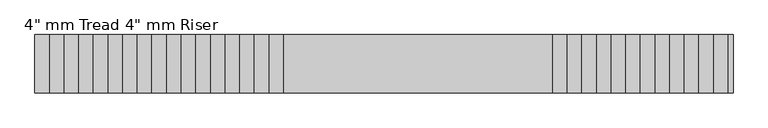
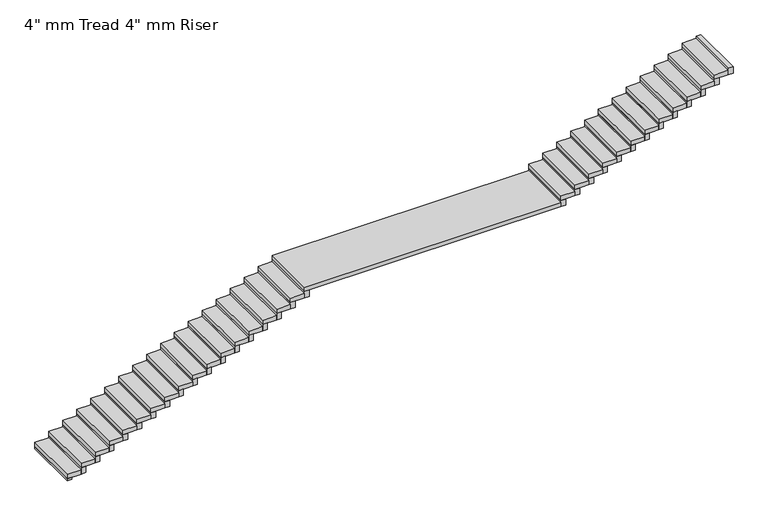
"""IFC4 building model written with IfcOpenShell, lengths in millimetres: stair flight geometry."""

from ifc_helpers import new_model, si_unit, frame, origin, origin_with_axes, place, context, project, spatial, polyline, outline, extrude, source, transform, mapped, element, save


def stair_flight_c4523bda(model_context):
    return source(origin(), model_context, "Body", "SweptSolid", [
        extrude(outline(polyline([(18088.5587563, -31336.2205555), (17986.9587563, -31336.2205555), (17986.9587563, -30117.0205555), (18088.5587563, -30117.0205555), (18088.5587563, -31336.2205555)])), origin_with_axes(), (0.0, 0.0, 1.0), 45.883871),
        extrude(outline(polyline([(18291.7587563, -30117.0205555), (18291.7587563, -31336.2205555), (17986.9587563, -31336.2205555), (17986.9587563, -30117.0205555), (18291.7587563, -30117.0205555)])), frame((0.0, 0.0, 45.883871), z_axis=(0.0, 0.0, 1.0), x_axis=(1.0, 0.0, 0.0)), (0.0, 0.0, 1.0), 101.6),
        extrude(outline(polyline([(18393.3587563, -31336.2205555), (18291.7587563, -31336.2205555), (18291.7587563, -30117.0205555), (18393.3587563, -30117.0205555), (18393.3587563, -31336.2205555)])), frame((0.0, 0.0, 45.883871), z_axis=(0.0, 0.0, 1.0), x_axis=(1.0, 0.0, 0.0)), (0.0, 0.0, 1.0), 147.483871),
        extrude(outline(polyline([(18596.5587563, -30117.0205555), (18596.5587563, -31336.2205555), (18291.7587563, -31336.2205555), (18291.7587563, -30117.0205555), (18596.5587563, -30117.0205555)])), frame((0.0, 0.0, 193.3677419), z_axis=(0.0, 0.0, 1.0), x_axis=(1.0, 0.0, 0.0)), (0.0, 0.0, 1.0), 101.6),
        extrude(outline(polyline([(18698.1587563, -31336.2205555), (18596.5587563, -31336.2205555), (18596.5587563, -30117.0205555), (18698.1587563, -30117.0205555), (18698.1587563, -31336.2205555)])), frame((0.0, 0.0, 193.3677419), z_axis=(0.0, 0.0, 1.0), x_axis=(1.0, 0.0, 0.0)), (0.0, 0.0, 1.0), 147.483871),
        extrude(outline(polyline([(18901.3587563, -30117.0205555), (18901.3587563, -31336.2205555), (18596.5587563, -31336.2205555), (18596.5587563, -30117.0205555), (18901.3587563, -30117.0205555)])), frame((0.0, 0.0, 340.8516129), z_axis=(0.0, 0.0, 1.0), x_axis=(1.0, 0.0, 0.0)), (0.0, 0.0, 1.0), 101.6),
        extrude(outline(polyline([(19002.9587563, -31336.2205555), (18901.3587563, -31336.2205555), (18901.3587563, -30117.0205555), (19002.9587563, -30117.0205555), (19002.9587563, -31336.2205555)])), frame((0.0, 0.0, 340.8516129), z_axis=(0.0, 0.0, 1.0), x_axis=(1.0, 0.0, 0.0)), (0.0, 0.0, 1.0), 147.483871),
        extrude(outline(polyline([(19206.1587563, -30117.0205555), (19206.1587563, -31336.2205555), (18901.3587563, -31336.2205555), (18901.3587563, -30117.0205555), (19206.1587563, -30117.0205555)])), frame((0.0, 0.0, 488.3354839), z_axis=(0.0, 0.0, 1.0), x_axis=(1.0, 0.0, 0.0)), (0.0, 0.0, 1.0), 101.6),
        extrude(outline(polyline([(19307.7587563, -31336.2205555), (19206.1587563, -31336.2205555), (19206.1587563, -30117.0205555), (19307.7587563, -30117.0205555), (19307.7587563, -31336.2205555)])), frame((0.0, 0.0, 488.3354839), z_axis=(0.0, 0.0, 1.0), x_axis=(1.0, 0.0, 0.0)), (0.0, 0.0, 1.0), 147.483871),
        extrude(outline(polyline([(19510.9587563, -30117.0205555), (19510.9587563, -31336.2205555), (19206.1587563, -31336.2205555), (19206.1587563, -30117.0205555), (19510.9587563, -30117.0205555)])), frame((0.0, 0.0, 635.8193548), z_axis=(0.0, 0.0, 1.0), x_axis=(1.0, 0.0, 0.0)), (0.0, 0.0, 1.0), 101.6),
        extrude(outline(polyline([(19612.5587563, -31336.2205555), (19510.9587563, -31336.2205555), (19510.9587563, -30117.0205555), (19612.5587563, -30117.0205555), (19612.5587563, -31336.2205555)])), frame((0.0, 0.0, 635.8193548), z_axis=(0.0, 0.0, 1.0), x_axis=(1.0, 0.0, 0.0)), (0.0, 0.0, 1.0), 147.483871),
        extrude(outline(polyline([(19815.7587563, -30117.0205555), (19815.7587563, -31336.2205555), (19510.9587563, -31336.2205555), (19510.9587563, -30117.0205555), (19815.7587563, -30117.0205555)])), frame((0.0, 0.0, 783.3032258), z_axis=(0.0, 0.0, 1.0), x_axis=(1.0, 0.0, 0.0)), (0.0, 0.0, 1.0), 101.6),
        extrude(outline(polyline([(19917.3587563, -31336.2205555), (19815.7587563, -31336.2205555), (19815.7587563, -30117.0205555), (19917.3587563, -30117.0205555), (19917.3587563, -31336.2205555)])), frame((0.0, 0.0, 783.3032258), z_axis=(0.0, 0.0, 1.0), x_axis=(1.0, 0.0, 0.0)), (0.0, 0.0, 1.0), 147.483871),
        extrude(outline(polyline([(20120.5587563, -30117.0205555), (20120.5587563, -31336.2205555), (19815.7587563, -31336.2205555), (19815.7587563, -30117.0205555), (20120.5587563, -30117.0205555)])), frame((0.0, 0.0, 930.7870968), z_axis=(0.0, 0.0, 1.0), x_axis=(1.0, 0.0, 0.0)), (0.0, 0.0, 1.0), 101.6),
        extrude(outline(polyline([(20222.1587563, -31336.2205555), (20120.5587563, -31336.2205555), (20120.5587563, -30117.0205555), (20222.1587563, -30117.0205555), (20222.1587563, -31336.2205555)])), frame((0.0, 0.0, 930.7870968), z_axis=(0.0, 0.0, 1.0), x_axis=(1.0, 0.0, 0.0)), (0.0, 0.0, 1.0), 147.483871),
        extrude(outline(polyline([(20425.3587563, -30117.0205555), (20425.3587563, -31336.2205555), (20120.5587563, -31336.2205555), (20120.5587563, -30117.0205555), (20425.3587563, -30117.0205555)])), frame((0.0, 0.0, 1078.2709677), z_axis=(0.0, 0.0, 1.0), x_axis=(1.0, 0.0, 0.0)), (0.0, 0.0, 1.0), 101.6),
        extrude(outline(polyline([(20526.9587563, -31336.2205555), (20425.3587563, -31336.2205555), (20425.3587563, -30117.0205555), (20526.9587563, -30117.0205555), (20526.9587563, -31336.2205555)])), frame((0.0, 0.0, 1078.2709677), z_axis=(0.0, 0.0, 1.0), x_axis=(1.0, 0.0, 0.0)), (0.0, 0.0, 1.0), 147.483871),
        extrude(outline(polyline([(20730.1587563, -30117.0205555), (20730.1587563, -31336.2205555), (20425.3587563, -31336.2205555), (20425.3587563, -30117.0205555), (20730.1587563, -30117.0205555)])), frame((0.0, 0.0, 1225.7548387), z_axis=(0.0, 0.0, 1.0), x_axis=(1.0, 0.0, 0.0)), (0.0, 0.0, 1.0), 101.6),
        extrude(outline(polyline([(20831.7587563, -31336.2205555), (20730.1587563, -31336.2205555), (20730.1587563, -30117.0205555), (20831.7587563, -30117.0205555), (20831.7587563, -31336.2205555)])), frame((0.0, 0.0, 1225.7548387), z_axis=(0.0, 0.0, 1.0), x_axis=(1.0, 0.0, 0.0)), (0.0, 0.0, 1.0), 147.483871),
        extrude(outline(polyline([(21034.9587563, -30117.0205555), (21034.9587563, -31336.2205555), (20730.1587563, -31336.2205555), (20730.1587563, -30117.0205555), (21034.9587563, -30117.0205555)])), frame((0.0, 0.0, 1373.2387097), z_axis=(0.0, 0.0, 1.0), x_axis=(1.0, 0.0, 0.0)), (0.0, 0.0, 1.0), 101.6),
        extrude(outline(polyline([(21136.5587563, -31336.2205555), (21034.9587563, -31336.2205555), (21034.9587563, -30117.0205555), (21136.5587563, -30117.0205555), (21136.5587563, -31336.2205555)])), frame((0.0, 0.0, 1373.2387097), z_axis=(0.0, 0.0, 1.0), x_axis=(1.0, 0.0, 0.0)), (0.0, 0.0, 1.0), 147.483871),
        extrude(outline(polyline([(21339.7587563, -30117.0205555), (21339.7587563, -31336.2205555), (21034.9587563, -31336.2205555), (21034.9587563, -30117.0205555), (21339.7587563, -30117.0205555)])), frame((0.0, 0.0, 1520.7225806), z_axis=(0.0, 0.0, 1.0), x_axis=(1.0, 0.0, 0.0)), (0.0, 0.0, 1.0), 101.6),
        extrude(outline(polyline([(21441.3587563, -31336.2205555), (21339.7587563, -31336.2205555), (21339.7587563, -30117.0205555), (21441.3587563, -30117.0205555), (21441.3587563, -31336.2205555)])), frame((0.0, 0.0, 1520.7225806), z_axis=(0.0, 0.0, 1.0), x_axis=(1.0, 0.0, 0.0)), (0.0, 0.0, 1.0), 147.483871),
        extrude(outline(polyline([(21644.5587563, -30117.0205555), (21644.5587563, -31336.2205555), (21339.7587563, -31336.2205555), (21339.7587563, -30117.0205555), (21644.5587563, -30117.0205555)])), frame((0.0, 0.0, 1668.2064516), z_axis=(0.0, 0.0, 1.0), x_axis=(1.0, 0.0, 0.0)), (0.0, 0.0, 1.0), 101.6),
        extrude(outline(polyline([(32528.4587563, -31336.2205555), (32426.8587563, -31336.2205555), (32426.8587563, -30117.0205555), (32528.4587563, -30117.0205555), (32528.4587563, -31336.2205555)])), frame((0.0, 0.0, 4322.916129), z_axis=(0.0, 0.0, 1.0), x_axis=(1.0, 0.0, 0.0)), (0.0, 0.0, 1.0), 147.483871),
        extrude(outline(polyline([(21746.1587563, -31336.2205555), (21644.5587563, -31336.2205555), (21644.5587563, -30117.0205555), (21746.1587563, -30117.0205555), (21746.1587563, -31336.2205555)])), frame((0.0, 0.0, 1668.2064516), z_axis=(0.0, 0.0, 1.0), x_axis=(1.0, 0.0, 0.0)), (0.0, 0.0, 1.0), 147.483871),
        extrude(outline(polyline([(21949.3587563, -30117.0205555), (21949.3587563, -31336.2205555), (21644.5587563, -31336.2205555), (21644.5587563, -30117.0205555), (21949.3587563, -30117.0205555)])), frame((0.0, 0.0, 1815.6903226), z_axis=(0.0, 0.0, 1.0), x_axis=(1.0, 0.0, 0.0)), (0.0, 0.0, 1.0), 101.6),
        extrude(outline(polyline([(22050.9587563, -31336.2205555), (21949.3587563, -31336.2205555), (21949.3587563, -30117.0205555), (22050.9587563, -30117.0205555), (22050.9587563, -31336.2205555)])), frame((0.0, 0.0, 1815.6903226), z_axis=(0.0, 0.0, 1.0), x_axis=(1.0, 0.0, 0.0)), (0.0, 0.0, 1.0), 147.483871),
        extrude(outline(polyline([(22254.1587563, -30117.0205555), (22254.1587563, -31336.2205555), (21949.3587563, -31336.2205555), (21949.3587563, -30117.0205555), (22254.1587563, -30117.0205555)])), frame((0.0, 0.0, 1963.1741935), z_axis=(0.0, 0.0, 1.0), x_axis=(1.0, 0.0, 0.0)), (0.0, 0.0, 1.0), 101.6),
        extrude(outline(polyline([(22355.7587563, -31336.2205555), (22254.1587563, -31336.2205555), (22254.1587563, -30117.0205555), (22355.7587563, -30117.0205555), (22355.7587563, -31336.2205555)])), frame((0.0, 0.0, 1963.1741935), z_axis=(0.0, 0.0, 1.0), x_axis=(1.0, 0.0, 0.0)), (0.0, 0.0, 1.0), 147.483871),
        extrude(outline(polyline([(22558.9587563, -30117.0205555), (22558.9587563, -31336.2205555), (22254.1587563, -31336.2205555), (22254.1587563, -30117.0205555), (22558.9587563, -30117.0205555)])), frame((0.0, 0.0, 2110.6580645), z_axis=(0.0, 0.0, 1.0), x_axis=(1.0, 0.0, 0.0)), (0.0, 0.0, 1.0), 101.6),
        extrude(outline(polyline([(22660.5587563, -31336.2205555), (22558.9587563, -31336.2205555), (22558.9587563, -30117.0205555), (22660.5587563, -30117.0205555), (22660.5587563, -31336.2205555)])), frame((0.0, 0.0, 2110.6580645), z_axis=(0.0, 0.0, 1.0), x_axis=(1.0, 0.0, 0.0)), (0.0, 0.0, 1.0), 147.483871),
        extrude(outline(polyline([(22863.7587563, -30117.0205555), (22863.7587563, -31336.2205555), (22558.9587563, -31336.2205555), (22558.9587563, -30117.0205555), (22863.7587563, -30117.0205555)])), frame((0.0, 0.0, 2258.1419355), z_axis=(0.0, 0.0, 1.0), x_axis=(1.0, 0.0, 0.0)), (0.0, 0.0, 1.0), 101.6),
        extrude(outline(polyline([(22965.3587563, -31336.2205555), (22863.7587563, -31336.2205555), (22863.7587563, -30117.0205555), (22965.3587563, -30117.0205555), (22965.3587563, -31336.2205555)])), frame((0.0, 0.0, 2258.1419355), z_axis=(0.0, 0.0, 1.0), x_axis=(1.0, 0.0, 0.0)), (0.0, 0.0, 1.0), 147.483871),
        extrude(outline(polyline([(23168.5587563, -30117.0205555), (23168.5587563, -31336.2205555), (22863.7587563, -31336.2205555), (22863.7587563, -30117.0205555), (23168.5587563, -30117.0205555)])), frame((0.0, 0.0, 2405.6258065), z_axis=(0.0, 0.0, 1.0), x_axis=(1.0, 0.0, 0.0)), (0.0, 0.0, 1.0), 101.6),
        extrude(outline(polyline([(23270.1587563, -31336.2205555), (23168.5587563, -31336.2205555), (23168.5587563, -30117.0205555), (23270.1587563, -30117.0205555), (23270.1587563, -31336.2205555)])), frame((0.0, 0.0, 2405.6258065), z_axis=(0.0, 0.0, 1.0), x_axis=(1.0, 0.0, 0.0)), (0.0, 0.0, 1.0), 147.483871),
        extrude(outline(polyline([(28769.2587563, -30117.0205555), (28769.2587563, -31336.2205555), (23168.5587563, -31336.2205555), (23168.5587563, -30117.0205555), (28769.2587563, -30117.0205555)])), frame((0.0, 0.0, 2553.1096774), z_axis=(0.0, 0.0, 1.0), x_axis=(1.0, 0.0, 0.0)), (0.0, 0.0, 1.0), 101.6),
        extrude(outline(polyline([(28870.8587563, -31336.2205555), (28769.2587563, -31336.2205555), (28769.2587563, -30117.0205555), (28870.8587563, -30117.0205555), (28870.8587563, -31336.2205555)])), frame((0.0, 0.0, 2553.1096774), z_axis=(0.0, 0.0, 1.0), x_axis=(1.0, 0.0, 0.0)), (0.0, 0.0, 1.0), 147.483871),
        extrude(outline(polyline([(29074.0587563, -30117.0205555), (29074.0587563, -31336.2205555), (28769.2587563, -31336.2205555), (28769.2587563, -30117.0205555), (29074.0587563, -30117.0205555)])), frame((0.0, 0.0, 2700.5935484), z_axis=(0.0, 0.0, 1.0), x_axis=(1.0, 0.0, 0.0)), (0.0, 0.0, 1.0), 101.6),
        extrude(outline(polyline([(29175.6587563, -31336.2205555), (29074.0587563, -31336.2205555), (29074.0587563, -30117.0205555), (29175.6587563, -30117.0205555), (29175.6587563, -31336.2205555)])), frame((0.0, 0.0, 2700.5935484), z_axis=(0.0, 0.0, 1.0), x_axis=(1.0, 0.0, 0.0)), (0.0, 0.0, 1.0), 147.483871),
        extrude(outline(polyline([(29378.8587563, -30117.0205555), (29378.8587563, -31336.2205555), (29074.0587563, -31336.2205555), (29074.0587563, -30117.0205555), (29378.8587563, -30117.0205555)])), frame((0.0, 0.0, 2848.0774194), z_axis=(0.0, 0.0, 1.0), x_axis=(1.0, 0.0, 0.0)), (0.0, 0.0, 1.0), 101.6),
        extrude(outline(polyline([(29480.4587563, -31336.2205555), (29378.8587563, -31336.2205555), (29378.8587563, -30117.0205555), (29480.4587563, -30117.0205555), (29480.4587563, -31336.2205555)])), frame((0.0, 0.0, 2848.0774194), z_axis=(0.0, 0.0, 1.0), x_axis=(1.0, 0.0, 0.0)), (0.0, 0.0, 1.0), 147.483871),
        extrude(outline(polyline([(29683.6587563, -30117.0205555), (29683.6587563, -31336.2205555), (29378.8587563, -31336.2205555), (29378.8587563, -30117.0205555), (29683.6587563, -30117.0205555)])), frame((0.0, 0.0, 2995.5612903), z_axis=(0.0, 0.0, 1.0), x_axis=(1.0, 0.0, 0.0)), (0.0, 0.0, 1.0), 101.6),
        extrude(outline(polyline([(29785.2587563, -31336.2205555), (29683.6587563, -31336.2205555), (29683.6587563, -30117.0205555), (29785.2587563, -30117.0205555), (29785.2587563, -31336.2205555)])), frame((0.0, 0.0, 2995.5612903), z_axis=(0.0, 0.0, 1.0), x_axis=(1.0, 0.0, 0.0)), (0.0, 0.0, 1.0), 147.483871),
        extrude(outline(polyline([(29988.4587563, -30117.0205555), (29988.4587563, -31336.2205555), (29683.6587563, -31336.2205555), (29683.6587563, -30117.0205555), (29988.4587563, -30117.0205555)])), frame((0.0, 0.0, 3143.0451613), z_axis=(0.0, 0.0, 1.0), x_axis=(1.0, 0.0, 0.0)), (0.0, 0.0, 1.0), 101.6),
        extrude(outline(polyline([(30090.0587563, -31336.2205555), (29988.4587563, -31336.2205555), (29988.4587563, -30117.0205555), (30090.0587563, -30117.0205555), (30090.0587563, -31336.2205555)])), frame((0.0, 0.0, 3143.0451613), z_axis=(0.0, 0.0, 1.0), x_axis=(1.0, 0.0, 0.0)), (0.0, 0.0, 1.0), 147.483871),
        extrude(outline(polyline([(30293.2587563, -30117.0205555), (30293.2587563, -31336.2205555), (29988.4587563, -31336.2205555), (29988.4587563, -30117.0205555), (30293.2587563, -30117.0205555)])), frame((0.0, 0.0, 3290.5290323), z_axis=(0.0, 0.0, 1.0), x_axis=(1.0, 0.0, 0.0)), (0.0, 0.0, 1.0), 101.6),
        extrude(outline(polyline([(30394.8587563, -31336.2205555), (30293.2587563, -31336.2205555), (30293.2587563, -30117.0205555), (30394.8587563, -30117.0205555), (30394.8587563, -31336.2205555)])), frame((0.0, 0.0, 3290.5290323), z_axis=(0.0, 0.0, 1.0), x_axis=(1.0, 0.0, 0.0)), (0.0, 0.0, 1.0), 147.483871),
        extrude(outline(polyline([(30598.0587563, -30117.0205555), (30598.0587563, -31336.2205555), (30293.2587563, -31336.2205555), (30293.2587563, -30117.0205555), (30598.0587563, -30117.0205555)])), frame((0.0, 0.0, 3438.0129032), z_axis=(0.0, 0.0, 1.0), x_axis=(1.0, 0.0, 0.0)), (0.0, 0.0, 1.0), 101.6),
        extrude(outline(polyline([(30699.6587563, -31336.2205555), (30598.0587563, -31336.2205555), (30598.0587563, -30117.0205555), (30699.6587563, -30117.0205555), (30699.6587563, -31336.2205555)])), frame((0.0, 0.0, 3438.0129032), z_axis=(0.0, 0.0, 1.0), x_axis=(1.0, 0.0, 0.0)), (0.0, 0.0, 1.0), 147.483871),
        extrude(outline(polyline([(30902.8587563, -30117.0205555), (30902.8587563, -31336.2205555), (30598.0587563, -31336.2205555), (30598.0587563, -30117.0205555), (30902.8587563, -30117.0205555)])), frame((0.0, 0.0, 3585.4967742), z_axis=(0.0, 0.0, 1.0), x_axis=(1.0, 0.0, 0.0)), (0.0, 0.0, 1.0), 101.6),
        extrude(outline(polyline([(31004.4587563, -31336.2205555), (30902.8587563, -31336.2205555), (30902.8587563, -30117.0205555), (31004.4587563, -30117.0205555), (31004.4587563, -31336.2205555)])), frame((0.0, 0.0, 3585.4967742), z_axis=(0.0, 0.0, 1.0), x_axis=(1.0, 0.0, 0.0)), (0.0, 0.0, 1.0), 147.483871),
        extrude(outline(polyline([(31207.6587563, -30117.0205555), (31207.6587563, -31336.2205555), (30902.8587563, -31336.2205555), (30902.8587563, -30117.0205555), (31207.6587563, -30117.0205555)])), frame((0.0, 0.0, 3732.9806452), z_axis=(0.0, 0.0, 1.0), x_axis=(1.0, 0.0, 0.0)), (0.0, 0.0, 1.0), 101.6),
        extrude(outline(polyline([(31309.2587563, -31336.2205555), (31207.6587563, -31336.2205555), (31207.6587563, -30117.0205555), (31309.2587563, -30117.0205555), (31309.2587563, -31336.2205555)])), frame((0.0, 0.0, 3732.9806452), z_axis=(0.0, 0.0, 1.0), x_axis=(1.0, 0.0, 0.0)), (0.0, 0.0, 1.0), 147.483871),
        extrude(outline(polyline([(31512.4587563, -30117.0205555), (31512.4587563, -31336.2205555), (31207.6587563, -31336.2205555), (31207.6587563, -30117.0205555), (31512.4587563, -30117.0205555)])), frame((0.0, 0.0, 3880.4645161), z_axis=(0.0, 0.0, 1.0), x_axis=(1.0, 0.0, 0.0)), (0.0, 0.0, 1.0), 101.6),
        extrude(outline(polyline([(31614.0587563, -31336.2205555), (31512.4587563, -31336.2205555), (31512.4587563, -30117.0205555), (31614.0587563, -30117.0205555), (31614.0587563, -31336.2205555)])), frame((0.0, 0.0, 3880.4645161), z_axis=(0.0, 0.0, 1.0), x_axis=(1.0, 0.0, 0.0)), (0.0, 0.0, 1.0), 147.483871),
        extrude(outline(polyline([(31817.2587563, -30117.0205555), (31817.2587563, -31336.2205555), (31512.4587563, -31336.2205555), (31512.4587563, -30117.0205555), (31817.2587563, -30117.0205555)])), frame((0.0, 0.0, 4027.9483871), z_axis=(0.0, 0.0, 1.0), x_axis=(1.0, 0.0, 0.0)), (0.0, 0.0, 1.0), 101.6),
        extrude(outline(polyline([(31918.8587563, -31336.2205555), (31817.2587563, -31336.2205555), (31817.2587563, -30117.0205555), (31918.8587563, -30117.0205555), (31918.8587563, -31336.2205555)])), frame((0.0, 0.0, 4027.9483871), z_axis=(0.0, 0.0, 1.0), x_axis=(1.0, 0.0, 0.0)), (0.0, 0.0, 1.0), 147.483871),
        extrude(outline(polyline([(32122.0587563, -30117.0205555), (32122.0587563, -31336.2205555), (31817.2587563, -31336.2205555), (31817.2587563, -30117.0205555), (32122.0587563, -30117.0205555)])), frame((0.0, 0.0, 4175.4322581), z_axis=(0.0, 0.0, 1.0), x_axis=(1.0, 0.0, 0.0)), (0.0, 0.0, 1.0), 101.6),
        extrude(outline(polyline([(32223.6587563, -31336.2205555), (32122.0587563, -31336.2205555), (32122.0587563, -30117.0205555), (32223.6587563, -30117.0205555), (32223.6587563, -31336.2205555)])), frame((0.0, 0.0, 4175.4322581), z_axis=(0.0, 0.0, 1.0), x_axis=(1.0, 0.0, 0.0)), (0.0, 0.0, 1.0), 147.483871),
        extrude(outline(polyline([(32426.8587563, -30117.0205555), (32426.8587563, -31336.2205555), (32122.0587563, -31336.2205555), (32122.0587563, -30117.0205555), (32426.8587563, -30117.0205555)])), frame((0.0, 0.0, 4322.916129), z_axis=(0.0, 0.0, 1.0), x_axis=(1.0, 0.0, 0.0)), (0.0, 0.0, 1.0), 101.6),
    ])


if __name__ == "__main__":
    model = new_model("IFC4")
    model_context = context("Model", 3, world=origin())
    ifc_project = project(units=[si_unit("LENGTHUNIT", "METRE", prefix="MILLI")], contexts=[model_context])
    site = spatial("IfcSite", under=ifc_project)
    building = spatial("IfcBuilding", under=site)
    placement = place(None, origin())
    stair_flight_shape = stair_flight_c4523bda(model_context)
    element("IfcStairFlight", 1, ObjectType="4\" mm Tread 4\" mm Riser", at=placement, inside=building, context=model_context, shape_type="MappedRepresentation", body=[
        mapped(stair_flight_shape, transform((0.0, 0.0, 0.0), x_axis=(1.0, 0.0, 0.0), y_axis=(0.0, 1.0, 0.0), z_axis=(0.0, 0.0, 1.0))),
    ])
    save(model, "model.ifc")
